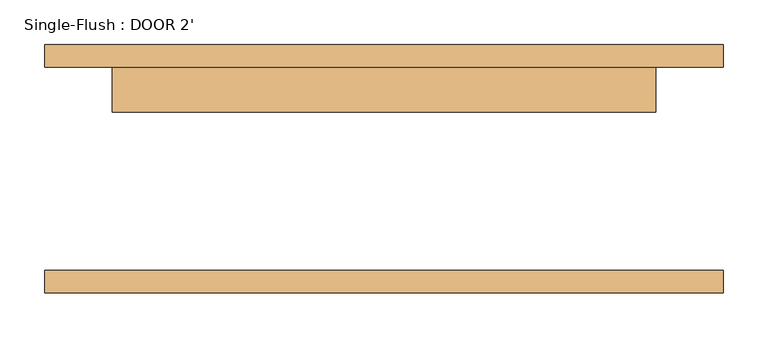
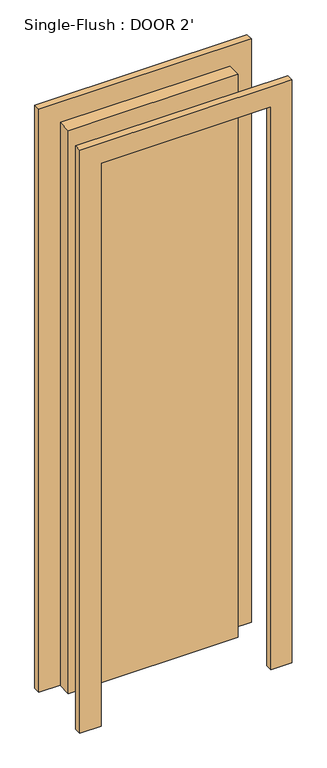
"""IFC4 building model written with IfcOpenShell, lengths in millimetres: door geometry, Single-Flush : DOOR 2'."""

from ifc_helpers import new_model, si_unit, frame, origin, origin_with_axes, place, context, project, spatial, polyline, outline, extrude, source, transform, mapped, element, save


def single_flush_door_2_0d3b4037(model_context):
    return source(origin(), model_context, "Body", "SweptSolid", [
        extrude(outline(polyline([(2209.8, -381.0), (0.0, -381.0), (0.0, -304.8), (2133.6, -304.8), (2133.6, 304.8), (0.0, 304.8), (0.0, 381.0), (2209.8, 381.0), (2209.8, -381.0)])), frame((0.0, 114.3, 0.0), z_axis=(0.0, 1.0, 0.0), x_axis=(0.0, 0.0, 1.0)), (0.0, 0.0, 1.0), 25.4),
        extrude(outline(polyline([(2209.8, 381.0), (2209.8, -381.0), (0.0, -381.0), (0.0, -304.8), (2133.6, -304.8), (2133.6, 304.8), (0.0, 304.8), (0.0, 381.0), (2209.8, 381.0)])), frame((0.0, -139.7, 0.0), z_axis=(0.0, 1.0, 0.0), x_axis=(0.0, 0.0, 1.0)), (0.0, 0.0, 1.0), 25.4),
        extrude(outline(polyline([(304.8, 63.5), (-304.8, 63.5), (-304.8, 114.3), (304.8, 114.3), (304.8, 63.5)])), origin_with_axes(), (0.0, 0.0, 1.0), 2133.6),
    ])


if __name__ == "__main__":
    model = new_model("IFC4")
    model_context = context("Model", 3, world=origin())
    ifc_project = project(units=[si_unit("LENGTHUNIT", "METRE", prefix="MILLI")], contexts=[model_context])
    site = spatial("IfcSite", under=ifc_project)
    building = spatial("IfcBuilding", under=site)
    placement = place(None, origin())
    single_flush_door_2_shape = single_flush_door_2_0d3b4037(model_context)
    element("IfcDoor", 1, ObjectType="Single-Flush : DOOR 2'", at=placement, inside=building, context=model_context, shape_type="MappedRepresentation", body=[
        mapped(single_flush_door_2_shape, transform((0.0, 0.0, 0.0), x_axis=(1.0, 0.0, 0.0), y_axis=(0.0, 1.0, 0.0), z_axis=(0.0, 0.0, 1.0))),
    ])
    save(model, "model.ifc")

# Revit data of these elements
# Type "Single-Flush : DOOR 2'"
#   Type Mark = "10"
#   Construction Type Id = "MDOOR"
#   Assembly Code = "C1020"
#   Analytic Construction = "Metal"
#   Thickness = 0' - 2"
#   Heat Transfer Coefficient (U) = 0.651978 BTU/(h·ft²·°F)
#   Height = 7' - 0"
#   Trim Projection Ext = 0' - 1"
#   Trim Projection Int = 0' - 1"
#   Trim Width = 0' - 3"
#   Width = 2' - 0"
#   Define Thermal Properties by = 1
#   Door Material = Door - Panel
#   Frame Material = Door - Frame
#   Visual Light Transmittance = 0
#   Solar Heat Gain Coefficient = 0
#   Function = (empty or 0)
#   Wall Closure = (empty or 0)
# Element 1 (IfcDoor, "Single-Flush : DOOR 2'")
#   Materials on its faces: "Door - Frame", "Door - Panel"
# Materials
#   "Door - Panel": class "Wood", colour RGB 210 159 95, transparency 0, Cost = 0
#   "Door - Frame": colour RGB 118 70 51, transparency 0, Cost = 0
